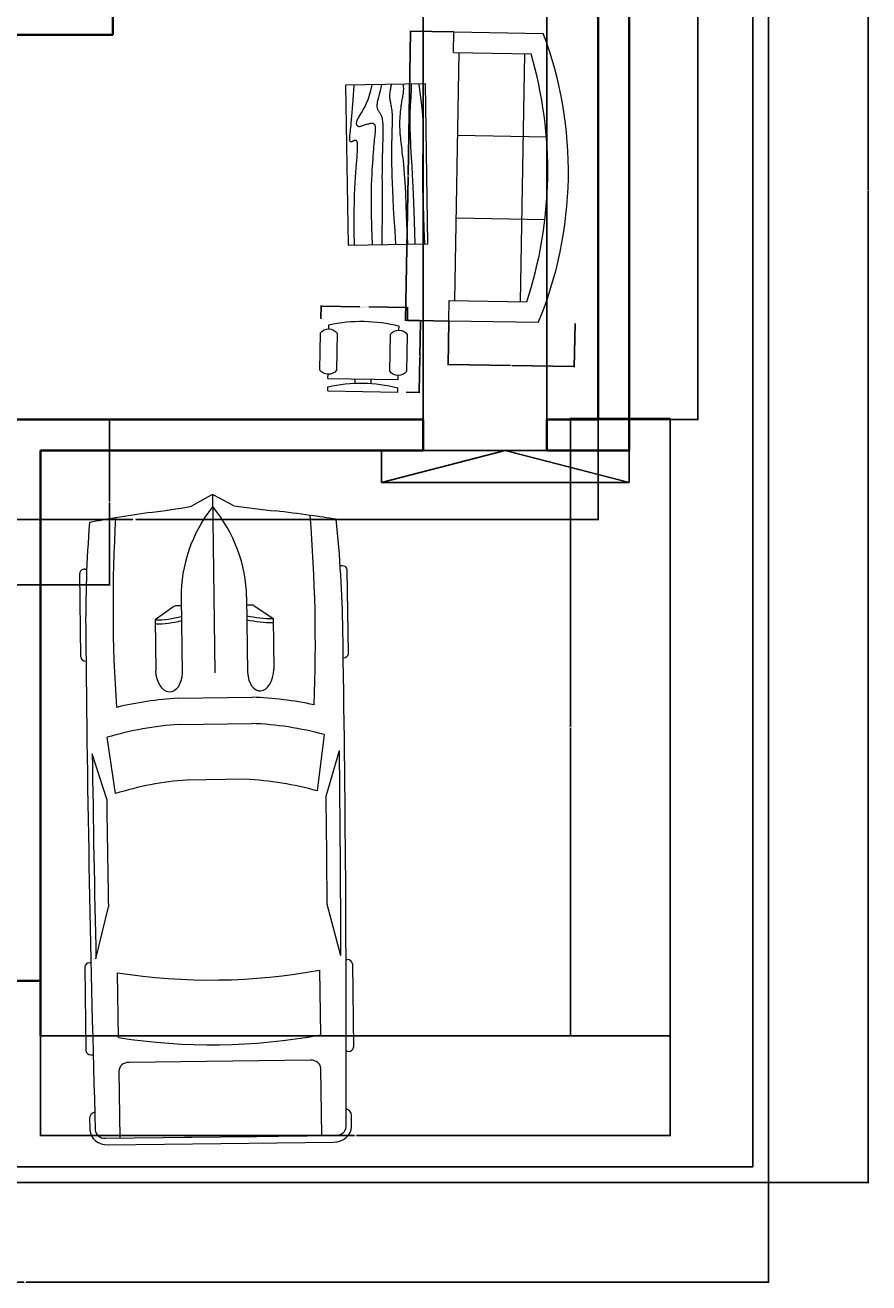
# Model space of a CAD drawing. Units: inches. Extents: x -1085 to 1941, y 1514 to 2348.
# Tile 3 of 9: x -613 to -367, y 1638 to 2003. Entities that reach past the tile are written whole.
import ezdxf

# ---------------------------------------------------------------- set-up
doc = ezdxf.new("R2010")
doc.units = ezdxf.units.IN
for name, color, linetype, lineweight in [('A-ANNO-DIMS', 2, 'Continuous', 18), ('A-FLOR-OTLN', 7, 'Continuous', 25), ('A-WALL', 7, 'Continuous', 35), ('C-PRKG-VEHS', 8, 'Continuous', 13), ('C-PROP', 8, 'Continuous', 25), ('FOUNITR-URE', 2, 'Continuous', 18)]:
    doc.layers.add(name, color=color, linetype=linetype, lineweight=lineweight)
doc.styles.get("Standard").update_dxf_attribs({"font": 'arial.ttf'})
doc.dimstyles.get("Standard").update_dxf_attribs({"dimtxt": 0.18, "dimasz": 0.18, "dimexe": 0.18, "dimexo": 0.0625, "dimgap": 0.09, "dimtad": 0, "dimtih": 1, "dimtoh": 1, "dimdec": 4, "dimzin": 0, "dimdsep": 46, "dimtxsty": 'Standard', "dimcen": 0.09, "dimadec": 0, "dimazin": 0, "dimtfac": 1, "dimtdec": 4, "dimtofl": 0, "dimtmove": 0, "dimatfit": 3, "dimfxl": 1, "dimtolj": 1, "dimtzin": 0, "dimarcsym": 0})

# ---------------------------------------------------------------- blocks, each defined once
blk = doc.blocks.new('Sofa - Roundback 7 ft.')
for p, q in [((-12.00002, -32.4421), (-12.00003, -6.5971)), ((11.99997, -32.4421), (11.99998, -6.5971)), ((-36.000027, -34), (-36.000027, -11.4696)), ((-35.999844, -13.3819), (35.9998, -13.3819)), ((35.99998, -34), (35.99998, -11.4696)), ((-36.000027, -32.4421), (35.99998, -32.4421))]:
    blk.add_line(p, q)
for points in [[(-36.000027, -34), (-42.000027, -34), (-42.000027, -8)], [(41.99998, -8), (41.99998, -34), (35.99998, -34)]]:
    blk.add_lwpolyline(points)
for centre, radius, start, end in [((0, -114.25), 114.25, 68.43141, 111.5686), ((-0.00001, -127.1968), 121.1968, 72.72033, 107.2797)]:
    blk.add_arc(centre, radius, start, end)
blk = doc.blocks.new('Chair - Desk')
for p, q in [((-8.5, 0), (-8.5, -1)), ((-8.5, 0), (8.5, 0)), ((8.5, 0), (8.5, -1)), ((-8.5, -3), (-8.5, -4)), ((-8.5, -3), (8.5, -3)), ((-2, -3), (-2, -1.9355)), ((2, -1.9576), (2, -3)), ((8.5, -3), (8.5, -4)), ((-10.5, -5), (-10.5, -14)), ((-6.5, -14), (-6.5, -5)), ((6.5, -5), (6.5, -14)), ((10.5, -14), (10.5, -5)), ((-8.5, -15), (-8.5, -16)), ((8.5, -15), (8.5, -16))]:
    blk.add_line(p, q)
for centre, radius, start, end in [((0, 34.625), 36.625, 256.5803, 283.4197), ((-8.5, -6.5), 2.5, 36.8699, 143.1301), ((8.5, -6.5), 2.5, 36.8699, 143.1301), ((-8.5, -12.5), 2.5, 216.8699, 323.1301), ((8.5, -12.5), 2.5, 216.8699, 323.1301), ((0, 19.625), 36.625, 256.5803, 283.4197)]:
    blk.add_arc(centre, radius, start, end)
blk = doc.blocks.new('*U28')
for p, q in [((536, 950.2), (536, 935.5)), ((1182.5, 987.8), (567.7, 987.8)), ((1214.1, 949.7), (1214.1, 950.2)), ((3440.5, 941.7), (3440.5, 950.2)), ((3472.1, 987.8), (4086.9, 987.8)), ((4118.5, 950.2), (4118.5, 934.1)), ((2234.8, 809.5), (1898.9, 912.4)), ((3411.6, 904.3), (3029.9, 807.2)), ((4736.4, -850.9), (4736.4, 850.9)), ((1778.8, 801), (2194.7, 745.5)), ((3515.9, 745.5), (3994.1, 745.5)), ((4736.4, 745.5), (4242, 745.5)), ((4785.3, -832.1), (4785.3, 832.1)), ((4178.7, 670.3), (4178.7, -670.3)), ((819.6, 295.3), (917.7, 436.1)), ((917.7, 436.1), (1293.8, 436.1)), ((815.9, 241.4), (815.9, 283.3)), ((756.2, 241.4), (1312.8, 241.4)), ((1496.5, -273.7), (1496.5, 273.7)), ((1690.4, -267.4), (1690.4, 267.4)), ((2101.5, 215.8), (2101.5, -215.8)), ((4736.4, -267.4), (4736.4, 267.4)), ((83, 155.7), (2.6, 10.3)), ((0, 0), (1312.8, 0)), ((2.6, -10.3), (83, -155.7)), ((756.2, -241.4), (1312.8, -241.4)), ((815.9, -241.4), (815.9, -283.3)), ((819.6, -295.3), (917.7, -436.1)), ((917.7, -436.1), (1293.8, -436.1)), ((2194.7, -745.5), (1778.8, -801)), ((2234.8, -809.5), (1898.9, -912.4)), ((3411.6, -904.3), (3029.9, -807.2)), ((3994.1, -745.5), (3515.9, -745.5)), ((4242, -745.5), (4736.4, -745.5)), ((536, -950.2), (536, -935.5)), ((1182.5, -987.8), (567.7, -987.8)), ((1214.1, -949.7), (1214.1, -950.2)), ((3440.5, -941.7), (3440.5, -950.2)), ((3472.1, -987.8), (4086.9, -987.8)), ((4118.5, -950.2), (4118.5, -934.1))]:
    blk.add_line(p, q)
for centre, major_axis, ratio, start_param, end_param in [((1046.3, -12467.9), (0, 13417.1), 0.842304, 0.00281, 0.075598), ((567.7, 950.2), (0, -37.6), 0.842304, 3.141593, 4.712389), ((1637.8, -268112.7), (0, 269062.9), 0.842304, -0.013397, 0.002797), ((1182.5, 950.2), (0, 37.6), 0.842304, -1.570796, 0), ((3472.1, 950.2), (0, -37.6), 0.842304, 3.141593, 4.712389), ((4086.9, 950.2), (0, 37.6), 0.842304, -1.570796, 0), ((4588, 910.3), (0, 56.4), 0.842304, -0.013017, 1.249894), ((1637.8, -268131.5), (0, 269121), 0.842304, -0.013397, -0.013017), ((4673.1, 832.1), (0, -133.3), 0.842304, 1.570796, 3.128196), ((6757.2, -699.1), (0, 7958), 0.842304, 1.367076, 1.39176), ((1637.8, -268112.7), (0, -269025.3), 0.842304, 3.133765, 3.140441), ((4673.1, 850.9), (0, -75.2), 0.842304, 1.570796, 3.128196), ((951.8, -15086.6), (0, -15832.5), 0.842304, 3.096046, 3.200911), ((3436.4, 136.8), (0, 2077), 0.842304, 1.245306, 1.50788), ((3799.7, 71.1), (0, -2021.3), 0.842304, 4.372215, 4.640744), ((2433, -93125.4), (0, -93935.2), 0.842304, 3.134049, 3.144098), ((433.9, 0), (0, 3734.3), 0.842304, 4.511394, 4.913384), ((912, 0), (0, 3734.3), 0.842304, 4.511394, 4.913384), ((4242, 670.3), (0, 75.2), 0.842304, 0, 1.570796), ((6583, -699.1), (0, -7754.7), 0.842304, 4.528606, 4.561838), ((3413.8, 136.8), (0, -2280.3), 0.842304, 4.449482, 4.652344), ((-5194.2, 1330.9), (0, -6374.4), 0.842304, 1.385369, 1.434372), ((331.1, 432), (0, 696.4), 0.842304, 4.435146, 4.718221), ((360.7, 432), (0, 696.4), 0.842304, 4.435146, 4.718221), ((1290.1, 338.8), (161, -9.1), 0.603834, -1.395552, 1.581315), ((831.8, 283.3), (0, 18.8), 0.842304, 0.879714, 1.570796), ((756.2, -1185.2), (0, 1426.7), 0.842304, 0, 0.590319), ((15.8, 0), (0, -18.8), 0.842304, 4.131459, 5.293319), ((756.2, 1185.2), (0, 1426.7), 0.842304, 2.551274, 3.141593), ((-5194.2, -1330.9), (0, 6374.4), 0.842304, -1.434372, -1.385369), ((331.1, -432), (0, -696.4), 0.842304, 1.564964, 1.848039), ((360.7, -432), (0, -696.4), 0.842304, 1.564964, 1.848039), ((3413.8, -136.8), (0, -2280.3), 0.842304, -1.510751, -1.307889), ((3436.4, -136.8), (0, -2077), 0.842304, -1.50788, -1.245306), ((3799.7, -71.1), (0, -2021.3), 0.842304, -1.499151, -1.230623), ((831.8, -283.3), (0, -18.8), 0.842304, 4.712389, 5.403472), ((6583, 699.1), (0, 7754.7), 0.842304, 1.721348, 1.754579), ((6757.2, 699.1), (0, 7958), 0.842304, 1.749832, 1.774517), ((951.8, 15086.6), (0, -15832.5), 0.842304, -0.059319, 0.045547), ((4242, -670.3), (0, -75.2), 0.842304, 4.712389, 6.283185), ((2433, 93125.4), (0, -93935.2), 0.842304, -0.002505, 0.007544), ((4673.1, -832.1), (0, -133.3), 0.842304, 0.013397, 1.570796), ((1046.3, 12467.9), (0, -13417.1), 0.842304, -0.075598, -0.00281), ((1637.8, 268112.7), (0, 269062.9), 0.842304, 3.138796, 3.15499), ((1637.8, 268112.7), (0, -269025.3), 0.842304, 0.001152, 0.007828), ((4673.1, -850.9), (0, 75.2), 0.842304, 3.15499, 4.712389), ((567.7, -950.2), (0, 37.6), 0.842304, 1.570796, 3.141593), ((1182.5, -950.2), (0, -37.6), 0.842304, 0, 1.570796), ((3472.1, -950.2), (0, -37.6), 0.842304, -1.570796, 0), ((4086.9, -950.2), (0, 37.6), 0.842304, 3.141593, 4.712389), ((4588, -910.3), (0, -56.4), 0.842304, -1.249894, 0.013017), ((1637.8, 268131.5), (0, 269121), 0.842304, 3.15461, 3.15499)]:
    blk.add_ellipse(centre, major_axis=major_axis, ratio=ratio, start_param=start_param, end_param=end_param)
at = {"extrusion": (0, 0, -1)}
blk.add_ellipse((1290.1, -338.8), major_axis=(161, 9.1), ratio=0.603834, start_param=-1.395552, end_param=1.581315, dxfattribs=at)
blk = doc.blocks.new('Table - Rectangular Woodgrain 60 x 30 in.')
for p, q in [((0, 0), (0, -30)), ((60, 0), (0, 0)), ((60, -30), (60, 0)), ((0, -30), (60, -30))]:
    blk.add_line(p, q)
for points in [[(0, -2.4), (4.8155, -2.418), (9.0302, -2.4688), (12.709, -2.5477), (15.9167, -2.65), (18.7181, -2.7711), (21.1781, -2.9063), (23.3616, -3.0508), (25.3333, -3.2), (27.1477, -3.3495), (28.8172, -3.4958), (30.3437, -3.636), (31.7291, -3.7667), (32.9756, -3.8849), (34.0849, -3.9875), (35.059, -4.0714), (35.9, -4.1334), (36.6114, -4.1711), (37.2041, -4.1854), (37.6906, -4.1779), (38.0833, -4.15), (38.3948, -4.1034), (38.6375, -4.0396), (38.8239, -3.9602), (38.9666, -3.8667), (39.0764, -3.7608), (39.1573, -3.6448), (39.2116, -3.521), (39.2416, -3.3917), (39.2498, -3.2593), (39.2385, -3.1261), (39.21, -2.9944), (39.1666, -2.8667), (39.111, -2.7447), (39.0468, -2.6281), (38.978, -2.5163), (38.9083, -2.4083), (38.8418, -2.3035), (38.7823, -2.201), (38.7337, -2.1001), (38.7, -2), (38.6844, -1.9003), (38.6875, -1.8021), (38.7094, -1.707), (38.75, -1.6167), (38.8094, -1.5326), (38.8875, -1.4563), (38.9844, -1.3893), (39.1, -1.3333), (39.2351, -1.2896), (39.3937, -1.2583), (39.5804, -1.2396), (39.8, -1.2333), (40.057, -1.2396), (40.3562, -1.2583), (40.7023, -1.2896), (41.1, -1.3333), (41.5547, -1.3895), (42.0755, -1.4573), (42.6721, -1.5361), (43.3542, -1.625), (44.1316, -1.7233), (45.014, -1.8302), (46.0114, -1.9449), (47.1333, -2.0667), (48.3862, -2.1947), (49.7625, -2.3281), (51.2513, -2.4663), (52.8416, -2.6083), (54.5226, -2.7535), (56.2833, -2.9011), (58.1127, -3.0501), (60, -3.2)], [(0, -9.2), (6.5759, -9.0858), (11.9385, -9.0365), (16.2527, -9.0418), (19.6833, -9.0917), (22.3952, -9.1759), (24.5531, -9.2844), (26.322, -9.4069), (27.8666, -9.5333), (29.3241, -9.6553), (30.7203, -9.7719), (32.0532, -9.8837), (33.3208, -9.9917), (34.5213, -10.0965), (35.6526, -10.199), (36.7128, -10.2999), (37.7, -10.4), (38.6129, -10.4996), (39.4531, -10.5969), (40.223, -10.6895), (40.925, -10.775), (41.5613, -10.8512), (42.1344, -10.9156), (42.6465, -10.966), (43.1, -11), (43.4976, -11.0158), (43.8437, -11.0136), (44.143, -10.9942), (44.4, -10.9583), (44.6195, -10.9069), (44.8062, -10.8406), (44.9648, -10.7603), (45.1, -10.6667), (45.2155, -10.5598), (45.3114, -10.4365), (45.3871, -10.2929), (45.4416, -10.125), (45.4743, -9.929), (45.4844, -9.7011), (45.4709, -9.4371), (45.4333, -9.1333), (45.3716, -8.7883), (45.2896, -8.4104), (45.1919, -8.0107), (45.0833, -7.6), (44.9685, -7.1893), (44.8521, -6.7896), (44.7388, -6.4117), (44.6333, -6.0667), (44.54, -5.7628), (44.4614, -5.4979), (44.4001, -5.2675), (44.3583, -5.0667), (44.3384, -4.8909), (44.3427, -4.7354), (44.3736, -4.5956), (44.4333, -4.4667), (44.5236, -4.3453), (44.6427, -4.2333), (44.7884, -4.1339), (44.9583, -4.05), (45.1501, -3.9849), (45.3614, -3.9417), (45.59, -3.9234), (45.8333, -3.9333), (46.0915, -3.9749), (46.3734, -4.0531), (46.6906, -4.1736), (47.0542, -4.3417), (47.4756, -4.5629), (47.9661, -4.8427), (48.5372, -5.1866), (49.2, -5.6), (49.9676, -6.0844), (50.8594, -6.625), (51.8965, -7.2031), (53.1, -7.8), (54.491, -8.3969), (56.0906, -8.975), (57.9199, -9.5156), (60, -10)], [(0, -12.8), (5.1847, -12.9322), (9.6213, -13.0323), (13.3963, -13.1059), (16.5958, -13.1583), (19.3063, -13.1952), (21.614, -13.2219), (23.6054, -13.2439), (25.3666, -13.2667), (26.9728, -13.2947), (28.4531, -13.3281), (29.8256, -13.3663), (31.1083, -13.4083), (32.3191, -13.4535), (33.476, -13.501), (34.597, -13.5501), (35.7, -13.6), (36.7984, -13.6497), (37.8875, -13.6979), (38.9578, -13.743), (40, -13.7833), (41.0047, -13.8174), (41.9625, -13.8438), (42.864, -13.8607), (43.7, -13.8667), (44.4631, -13.8604), (45.1552, -13.8417), (45.7801, -13.8104), (46.3416, -13.7667), (46.8439, -13.7104), (47.2906, -13.6417), (47.6858, -13.5604), (48.0333, -13.4667), (48.3375, -13.3608), (48.6042, -13.2448), (48.8396, -13.121), (49.05, -12.9917), (49.2417, -12.8593), (49.4208, -12.7261), (49.5937, -12.5944), (49.7667, -12.4667), (49.9452, -12.3451), (50.1323, -12.2313), (50.3303, -12.1268), (50.5416, -12.0333), (50.7686, -11.9524), (51.0135, -11.8854), (51.2788, -11.8341), (51.5666, -11.8), (51.8785, -11.7843), (52.2116, -11.7865), (52.562, -11.8059), (52.926, -11.8417), (53.2998, -11.8931), (53.6795, -11.9594), (54.0614, -12.0397), (54.4416, -12.1333), (54.8223, -12.2401), (55.2293, -12.3625), (55.6942, -12.5037), (56.2489, -12.6667), (56.9251, -12.8547), (57.7545, -13.0708), (58.7689, -13.3182), (60, -13.6)], [(0, -18), (5.124, -17.7273), (9.6609, -17.5057), (13.6705, -17.3303), (17.2125, -17.1958), (20.3467, -17.0973), (23.1328, -17.0297), (25.6307, -16.9878), (27.9, -16.9667), (29.9928, -16.9617), (31.9302, -16.9703), (33.7254, -16.9907), (35.3917, -17.0208), (36.9423, -17.0588), (38.3906, -17.1026), (39.7499, -17.1503), (41.0333, -17.2), (42.2519, -17.2496), (43.4073, -17.2969), (44.4986, -17.3395), (45.525, -17.375), (46.4858, -17.4012), (47.3802, -17.4156), (48.2074, -17.416), (48.9667, -17.4), (49.6583, -17.3662), (50.2872, -17.3167), (50.8595, -17.2547), (51.3812, -17.1833), (51.8584, -17.1057), (52.2971, -17.025), (52.7034, -16.9443), (53.0833, -16.8667), (53.443, -16.7951), (53.789, -16.7313), (54.128, -16.6768), (54.4666, -16.6334), (54.8115, -16.6024), (55.1693, -16.5854), (55.5465, -16.5841), (55.95, -16.6), (56.3828, -16.6337), (56.8346, -16.6823), (57.2915, -16.7418), (57.7396, -16.8084), (58.165, -16.878), (58.5539, -16.9469), (58.8924, -17.0111), (59.1666, -17.0667), (59.3679, -17.1107), (59.5078, -17.1438), (59.6032, -17.1675), (59.6708, -17.1833), (59.7275, -17.193), (59.7901, -17.1979), (59.8753, -17.1998), (60, -17.2)], [(0, -22.4), (8.0098, -22.2501), (14.4094, -22.1011), (19.4168, -21.9535), (23.25, -21.8083), (26.1269, -21.6663), (28.2656, -21.5281), (29.884, -21.3947), (31.2, -21.2667), (32.3967, -21.1448), (33.5172, -21.0292), (34.5697, -20.9198), (35.5625, -20.8167), (36.5037, -20.7198), (37.4015, -20.6292), (38.2642, -20.5448), (39.1, -20.4667), (39.9164, -20.3951), (40.7187, -20.3313), (41.5117, -20.2768), (42.3, -20.2333), (43.0883, -20.2024), (43.8812, -20.1854), (44.6836, -20.1841), (45.5, -20.2), (46.3328, -20.234), (47.1747, -20.2844), (48.0163, -20.3488), (48.8479, -20.425), (49.66, -20.5106), (50.4429, -20.6031), (51.1872, -20.7004), (51.8833, -20.8), (52.5246, -20.8999), (53.1166, -20.9995), (53.6681, -21.0983), (54.1875, -21.1958), (54.6834, -21.2919), (55.1646, -21.3859), (55.6394, -21.4777), (56.1167, -21.5667), (56.6028, -21.6515), (57.0961, -21.7266), (57.5929, -21.7852), (58.0896, -21.8208), (58.5823, -21.8268), (59.0674, -21.7964), (59.5412, -21.723), (60, -21.6)], [(0, -25.2), (8.6355, -25.0504), (15.7026, -24.9031), (21.4049, -24.7606), (25.9458, -24.625), (29.529, -24.4988), (32.3578, -24.3844), (34.6359, -24.284), (36.5667, -24.2), (38.3213, -24.1341), (39.9417, -24.0854), (41.437, -24.0523), (42.8167, -24.0333), (44.0901, -24.0268), (45.2667, -24.0313), (46.3557, -24.0451), (47.3667, -24.0667), (48.309, -24.0947), (49.1928, -24.1287), (50.0284, -24.168), (50.826, -24.2125), (51.5959, -24.2617), (52.3483, -24.3151), (53.0935, -24.3725), (53.8417, -24.4334), (54.6009, -24.497), (55.3699, -24.561), (56.1454, -24.6226), (56.9239, -24.6792), (57.7021, -24.7279), (58.4764, -24.7662), (59.2435, -24.7911), (60, -24.8)], [(0, -28.8), (5.6867, -28.6681), (10.45, -28.5698), (14.407, -28.5012), (17.675, -28.4584), (20.3711, -28.4374), (22.6125, -28.4344), (24.5164, -28.4455), (26.2, -28.4667), (27.762, -28.4947), (29.2276, -28.5281), (30.6033, -28.5663), (31.8958, -28.6084), (33.1118, -28.6535), (34.2578, -28.7011), (35.3405, -28.7501), (36.3666, -28.8), (37.3443, -28.8497), (38.288, -28.8974), (39.2137, -28.9412), (40.1375, -28.9792), (41.0753, -29.0093), (42.0432, -29.0297), (43.0572, -29.0384), (44.1333, -29.0333), (45.2936, -29.0114), (46.5843, -28.9641), (48.0579, -28.8816), (49.7666, -28.7542), (51.7629, -28.5721), (54.0989, -28.3255), (56.8272, -28.0048), (60, -27.6)]]:
    blk.add_lwpolyline(points)
blk = doc.blocks.new('*D42')
at = {"layer": 'A-ANNO-DIMS', "color": 0, "lineweight": -2, "transparency": 16777216}
for p, q in [((-500.6, 2001.04), (-501.33, 1959.41)), ((-488.06, 2001), (-500.78, 2001.22)), ((-502.05, 1917.41), (-501.33, 1959.04)), ((-489.52, 1917.01), (-502.24, 1917.23))]:
    blk.add_line(p, q, dxfattribs=at)
at = {"layer": 'A-ANNO-DIMS', "color": 0, "transparency": 16777216}
for points in [[(-500.63, 2001.04), (-500.57, 2001.04), (-500.6, 2001.22)], [(-502.08, 1917.41), (-502.02, 1917.41), (-502.06, 1917.23)]]:
    blk.add_solid(points, dxfattribs=at)
at = {"layer": 'Defpoints', "color": 0, "transparency": 16777216}
for p in [(-488, 2001), (-502.06, 1917.23), (-489.46, 1917.01)]:
    blk.add_point(p, dxfattribs=at)
at = {"layer": 'A-ANNO-DIMS', "color": 0, "transparency": 16777216, "insert": (-501.33, 1959.22), "char_height": 0.18, "attachment_point": 5}
blk.add_mtext('\\A1;SOFA 84', dxfattribs=at)
blk = doc.blocks.new('*D43')
at = {"layer": 'A-ANNO-DIMS', "color": 0, "lineweight": -2, "transparency": 16777216}
for p, q in [((-489.46, 1916.95), (-489.68, 1904.23)), ((-452.8, 1916.31), (-453.02, 1903.6)), ((-489.5, 1904.41), (-471.57, 1904.1)), ((-453.2, 1903.78), (-471.13, 1904.09))]:
    blk.add_line(p, q, dxfattribs=at)
at = {"layer": 'A-ANNO-DIMS', "color": 0, "transparency": 16777216}
for points in [[(-489.5, 1904.44), (-489.5, 1904.38), (-489.68, 1904.41)], [(-453.2, 1903.81), (-453.2, 1903.75), (-453.02, 1903.78)]]:
    blk.add_solid(points, dxfattribs=at)
at = {"layer": 'Defpoints', "color": 0, "transparency": 16777216}
for p in [(-489.46, 1917.01), (-452.8, 1916.37), (-453.02, 1903.78)]:
    blk.add_point(p, dxfattribs=at)
at = {"layer": 'A-ANNO-DIMS', "color": 0, "transparency": 16777216, "insert": (-471.35, 1904.09), "char_height": 0.18, "attachment_point": 5}
blk.add_mtext('\\A1;37', dxfattribs=at)
blk = doc.blocks.new('*D56')
at = {"layer": 'A-ANNO-DIMS', "color": 0, "lineweight": -2, "transparency": 16777216}
for p, q in [((-526.68, 1917.64), (-526.61, 1921.53)), ((-526.43, 1921.35), (-515.36, 1921.15)), ((-501.63, 1920.91), (-512.7, 1921.1)), ((-501.51, 1917.19), (-501.45, 1921.08))]:
    blk.add_line(p, q, dxfattribs=at)
at = {"layer": 'A-ANNO-DIMS', "color": 0, "transparency": 16777216}
for points in [[(-526.43, 1921.38), (-526.43, 1921.32), (-526.61, 1921.35)], [(-501.63, 1920.94), (-501.63, 1920.88), (-501.45, 1920.9)]]:
    blk.add_solid(points, dxfattribs=at)
at = {"layer": 'Defpoints', "color": 0, "transparency": 16777216}
for p in [(-526.68, 1917.58), (-501.45, 1920.9), (-501.52, 1917.13)]:
    blk.add_point(p, dxfattribs=at)
at = {"layer": 'A-ANNO-DIMS', "color": 0, "transparency": 16777216, "insert": (-514.03, 1921.13), "char_height": 0.18, "attachment_point": 5}
blk.add_mtext('\\A1;DESK CHAIR 25 TYP.', dxfattribs=at)
blk = doc.blocks.new('*D57')
at = {"layer": 'A-ANNO-DIMS', "color": 0, "lineweight": -2, "transparency": 16777216}
for p, q in [((-501.45, 1917.13), (-497.56, 1917.06)), ((-497.74, 1916.88), (-497.92, 1906.86)), ((-498.11, 1896.47), (-497.93, 1906.5)), ((-501.82, 1896.36), (-497.93, 1896.29))]:
    blk.add_line(p, q, dxfattribs=at)
at = {"layer": 'A-ANNO-DIMS', "color": 0, "transparency": 16777216}
for points in [[(-497.77, 1916.88), (-497.71, 1916.88), (-497.74, 1917.06)], [(-498.14, 1896.47), (-498.08, 1896.47), (-498.11, 1896.29)]]:
    blk.add_solid(points, dxfattribs=at)
at = {"layer": 'Defpoints', "color": 0, "transparency": 16777216}
for p in [(-501.52, 1917.13), (-501.88, 1896.36), (-498.11, 1896.29)]:
    blk.add_point(p, dxfattribs=at)
at = {"layer": 'A-ANNO-DIMS', "color": 0, "transparency": 16777216, "insert": (-497.93, 1906.68), "char_height": 0.18, "attachment_point": 5}
blk.add_mtext('\\A1;21 TYP.', dxfattribs=at)
blk = doc.blocks.new('*D94')
at = {"layer": 'A-ANNO-DIMS', "color": 0, "lineweight": -2, "transparency": 16777216}
for p, q in [((-828.6, 1666.82), (-828.6, 1637.7)), ((-396.6, 1666.82), (-396.6, 1637.7)), ((-828.42, 1637.88), (-612.89, 1637.88)), ((-396.78, 1637.88), (-612.31, 1637.88))]:
    blk.add_line(p, q, dxfattribs=at)
at = {"layer": 'A-ANNO-DIMS', "color": 0, "transparency": 16777216}
for points in [[(-828.42, 1637.91), (-828.42, 1637.85), (-828.6, 1637.88)], [(-396.78, 1637.91), (-396.78, 1637.85), (-396.6, 1637.88)]]:
    blk.add_solid(points, dxfattribs=at)
at = {"layer": 'Defpoints', "color": 0, "transparency": 16777216}
for p in [(-828.6, 1666.88), (-396.6, 1666.88), (-396.6, 1637.88)]:
    blk.add_point(p, dxfattribs=at)
at = {"layer": 'A-ANNO-DIMS', "color": 0, "transparency": 16777216, "insert": (-612.6, 1637.88), "char_height": 0.18, "attachment_point": 5}
blk.add_mtext('\\A1;432', dxfattribs=at)
blk = doc.blocks.new('*D95')
at = {"layer": 'A-ANNO-DIMS', "color": 0, "lineweight": -2, "transparency": 16777216}
for p, q in [((-396.54, 2242.88), (-367.42, 2242.88)), ((-367.6, 2242.7), (-367.6, 1955.07)), ((-367.6, 1667.06), (-367.6, 1954.7)), ((-396.54, 1666.88), (-367.42, 1666.88))]:
    blk.add_line(p, q, dxfattribs=at)
at = {"layer": 'A-ANNO-DIMS', "color": 0, "transparency": 16777216}
for points in [[(-367.63, 2242.7), (-367.57, 2242.7), (-367.6, 2242.88)], [(-367.63, 1667.06), (-367.57, 1667.06), (-367.6, 1666.88)]]:
    blk.add_solid(points, dxfattribs=at)
at = {"layer": 'Defpoints', "color": 0, "transparency": 16777216}
for p in [(-396.6, 2242.88), (-367.6, 2242.88), (-396.6, 1666.88)]:
    blk.add_point(p, dxfattribs=at)
at = {"layer": 'A-ANNO-DIMS', "color": 0, "transparency": 16777216, "insert": (-367.6, 1954.88), "char_height": 0.18, "attachment_point": 5}
blk.add_mtext('\\A1;576', dxfattribs=at)
blk = doc.blocks.new('*D108')
at = {"layer": 'A-ANNO-DIMS', "color": 0, "lineweight": -2, "transparency": 16777216}
for p, q in [((-496.94, 1888.45), (-496.94, 2272.06)), ((-496.76, 2271.88), (-479.16, 2271.88)), ((-461.12, 2271.88), (-478.72, 2271.88)), ((-460.94, 1888.45), (-460.94, 2272.06))]:
    blk.add_line(p, q, dxfattribs=at)
at = {"layer": 'A-ANNO-DIMS', "color": 0, "transparency": 16777216}
for points in [[(-496.76, 2271.91), (-496.76, 2271.85), (-496.94, 2271.88)], [(-461.12, 2271.91), (-461.12, 2271.85), (-460.94, 2271.88)]]:
    blk.add_solid(points, dxfattribs=at)
at = {"layer": 'Defpoints', "color": 0, "transparency": 16777216}
for p in [(-460.94, 2271.88), (-496.94, 1888.38), (-460.94, 1888.38)]:
    blk.add_point(p, dxfattribs=at)
at = {"layer": 'A-ANNO-DIMS', "color": 0, "transparency": 16777216, "insert": (-478.94, 2271.88), "char_height": 0.18, "attachment_point": 5}
blk.add_mtext('\\A1;36', dxfattribs=at)
blk = doc.blocks.new('*D110')
at = {"layer": 'A-ANNO-DIMS', "color": 0, "lineweight": -2, "transparency": 16777216}
for p, q in [((-446.04, 2196.38), (-416.92, 2196.38)), ((-417.1, 2196.2), (-417.1, 2042.57)), ((-417.1, 1888.56), (-417.1, 2042.2)), ((-446.04, 1888.38), (-416.92, 1888.38))]:
    blk.add_line(p, q, dxfattribs=at)
at = {"layer": 'A-ANNO-DIMS', "color": 0, "transparency": 16777216}
for points in [[(-417.13, 2196.2), (-417.07, 2196.2), (-417.1, 2196.38)], [(-417.13, 1888.56), (-417.07, 1888.56), (-417.1, 1888.38)]]:
    blk.add_solid(points, dxfattribs=at)
at = {"layer": 'Defpoints', "color": 0, "transparency": 16777216}
for p in [(-446.1, 2196.38), (-446.1, 1888.38), (-417.1, 1888.38)]:
    blk.add_point(p, dxfattribs=at)
at = {"layer": 'A-ANNO-DIMS', "color": 0, "transparency": 16777216, "insert": (-417.1, 2042.38), "char_height": 0.18, "attachment_point": 5}
blk.add_mtext('\\A1;308', dxfattribs=at)
blk = doc.blocks.new('*D112')
at = {"layer": 'A-ANNO-DIMS', "color": 0, "lineweight": -2, "transparency": 16777216}
for p, q in [((-715.62, 1888.32), (-715.62, 1859.2)), ((-446.1, 1888.32), (-446.1, 1859.2)), ((-715.44, 1859.38), (-581.26, 1859.38)), ((-446.28, 1859.38), (-580.47, 1859.38))]:
    blk.add_line(p, q, dxfattribs=at)
at = {"layer": 'A-ANNO-DIMS', "color": 0, "transparency": 16777216}
for points in [[(-715.44, 1859.41), (-715.44, 1859.35), (-715.62, 1859.38)], [(-446.28, 1859.41), (-446.28, 1859.35), (-446.1, 1859.38)]]:
    blk.add_solid(points, dxfattribs=at)
at = {"layer": 'Defpoints', "color": 0, "transparency": 16777216}
for p in [(-715.62, 1888.38), (-446.1, 1888.38), (-715.62, 1859.38)]:
    blk.add_point(p, dxfattribs=at)
at = {"layer": 'A-ANNO-DIMS', "color": 0, "transparency": 16777216, "insert": (-580.86, 1859.38), "char_height": 0.18, "attachment_point": 5}
blk.add_mtext('\\A1;269.5', dxfattribs=at)
blk = doc.blocks.new('*D113')
at = {"layer": 'A-ANNO-DIMS', "color": 0, "lineweight": -2, "transparency": 16777216}
for p, q in [((-608.1, 1709.42), (-608.1, 1680.3)), ((-425.1, 1709.42), (-425.1, 1680.3)), ((-607.92, 1680.48), (-516.88, 1680.48)), ((-425.28, 1680.48), (-516.32, 1680.48))]:
    blk.add_line(p, q, dxfattribs=at)
at = {"layer": 'A-ANNO-DIMS', "color": 0, "transparency": 16777216}
for points in [[(-607.92, 1680.51), (-607.92, 1680.45), (-608.1, 1680.48)], [(-425.28, 1680.51), (-425.28, 1680.45), (-425.1, 1680.48)]]:
    blk.add_solid(points, dxfattribs=at)
at = {"layer": 'Defpoints', "color": 0, "transparency": 16777216}
for p in [(-608.1, 1709.48), (-425.1, 1709.48), (-608.1, 1680.48)]:
    blk.add_point(p, dxfattribs=at)
at = {"layer": 'A-ANNO-DIMS', "color": 0, "transparency": 16777216, "insert": (-516.6, 1680.48), "char_height": 0.18, "attachment_point": 5}
blk.add_mtext('\\A1;183', dxfattribs=at)
blk = doc.blocks.new('*D114')
at = {"layer": 'A-ANNO-DIMS', "color": 0, "lineweight": -2, "transparency": 16777216}
for p, q in [((-425.17, 1888.71), (-454.28, 1888.71)), ((-454.1, 1888.53), (-454.1, 1799.28)), ((-454.1, 1709.66), (-454.1, 1798.91)), ((-425.17, 1709.48), (-454.28, 1709.48))]:
    blk.add_line(p, q, dxfattribs=at)
at = {"layer": 'A-ANNO-DIMS', "color": 0, "transparency": 16777216}
for points in [[(-454.13, 1888.53), (-454.07, 1888.53), (-454.1, 1888.71)], [(-454.13, 1709.66), (-454.07, 1709.66), (-454.1, 1709.48)]]:
    blk.add_solid(points, dxfattribs=at)
at = {"layer": 'Defpoints', "color": 0, "transparency": 16777216}
for p in [(-454.1, 1888.71), (-425.1, 1888.71), (-425.1, 1709.48)]:
    blk.add_point(p, dxfattribs=at)
at = {"layer": 'A-ANNO-DIMS', "color": 0, "transparency": 16777216, "insert": (-454.1, 1799.09), "char_height": 0.18, "attachment_point": 5}
blk.add_mtext('\\A1;179.23', dxfattribs=at)
blk = doc.blocks.new('*D118')
at = {"layer": 'A-ANNO-DIMS', "color": 0, "lineweight": -2, "transparency": 16777216}
for p, q in [((-617.04, 1888.38), (-587.92, 1888.38)), ((-588.1, 1888.2), (-588.1, 1864.57)), ((-588.1, 1840.56), (-588.1, 1864.2)), ((-617.04, 1840.38), (-587.92, 1840.38))]:
    blk.add_line(p, q, dxfattribs=at)
at = {"layer": 'A-ANNO-DIMS', "color": 0, "transparency": 16777216}
for points in [[(-588.13, 1888.2), (-588.07, 1888.2), (-588.1, 1888.38)], [(-588.13, 1840.56), (-588.07, 1840.56), (-588.1, 1840.38)]]:
    blk.add_solid(points, dxfattribs=at)
at = {"layer": 'Defpoints', "color": 0, "transparency": 16777216}
for p in [(-617.1, 1888.38), (-617.1, 1840.38), (-588.1, 1840.38)]:
    blk.add_point(p, dxfattribs=at)
at = {"layer": 'A-ANNO-DIMS', "color": 0, "transparency": 16777216, "insert": (-588.1, 1864.38), "char_height": 0.18, "attachment_point": 5}
blk.add_mtext('\\A1;48', dxfattribs=at)

msp = doc.modelspace()

# ---------------------------------------------------------------- linework, layer by layer
at = {"layer": 'A-FLOR-OTLN'}
for p, q in [((-425.1032, 1888.7098), (-437.1032, 1888.7098)), ((-425.1032, 1879.3835), (-425.1032, 1888.7098)), ((-437.1032, 1879.3835), (-509.0632, 1879.3835)), ((-509.0632, 1879.3835), (-509.0632, 1870.0845)), ((-473.0832, 1879.3835), (-509.0632, 1870.0845)), ((-509.0632, 1870.0845), (-473.0832, 1879.3835)), ((-473.0832, 1879.3835), (-437.1032, 1870.0845)), ((-437.1032, 1879.3835), (-437.1032, 1870.0845)), ((-425.1032, 1709.4784), (-425.1032, 1879.3835)), ((-509.0632, 1870.0845), (-437.4691, 1870.0845)), ((-437.4691, 1870.0845), (-437.1032, 1870.0845)), ((-437.1032, 1709.4784), (-608.1032, 1709.4784)), ((-437.1032, 1709.4784), (-425.1032, 1709.4784)), ((-608.1032, 1671.3835), (-608.1032, 1671.3835))]:
    msp.add_line(p, q, dxfattribs=at)
at = {"layer": 'A-WALL'}
for p, q in [((-437.1032, 2205.3835), (-437.1032, 1888.7098)), ((-446.1032, 2196.3835), (-446.1032, 1888.3835)), ((-587.1032, 2000.1777), (-587.1032, 2129.054)), ((-645.6032, 2000.1777), (-591.6032, 2000.1777)), ((-591.6032, 2000.1777), (-587.1032, 2000.1777)), ((-617.1032, 1888.3835), (-496.941, 1888.3835)), ((-496.941, 1879.3835), (-496.941, 1888.3835)), ((-460.941, 1888.3835), (-460.941, 1879.3835)), ((-460.941, 1888.3835), (-446.1032, 1888.3835)), ((-437.1032, 1888.7098), (-437.1032, 1879.3835)), ((-608.1032, 1709.4784), (-608.1032, 1879.3835)), ((-608.1032, 1879.3835), (-496.941, 1879.3835)), ((-460.941, 1879.3835), (-446.1032, 1879.3835)), ((-446.1032, 1879.3835), (-437.1032, 1879.3835)), ((-608.1032, 1734.3835), (-608.1032, 1709.4784)), ((-608.1032, 1725.3835), (-791.1032, 1725.3835)), ((-608.1032, 1725.3835), (-608.1032, 1709.4784))]:
    msp.add_line(p, q, dxfattribs=at)
at = {"layer": 'C-PROP'}
for p, q in [((-396.6032, 2242.8835), (-396.6032, 1666.8835)), ((-401.1032, 2238.3835), (-401.1032, 1671.3835)), ((-401.1032, 1671.3835), (-824.1032, 1671.3835)), ((-396.6032, 1666.8835), (-828.6032, 1666.8835))]:
    msp.add_line(p, q, dxfattribs=at)

# ---------------------------------------------------------------- block references
at = {"layer": 'C-PRKG-VEHS', "xscale": 0.0393700787401575, "yscale": 0.0393700787401575, "zscale": 0.0393700787401575, "rotation": 270.7362034403327}
msp.add_blockref('*U28', (-558.1441, 1866.5654), dxfattribs=at)
at = {"layer": 'FOUNITR-URE', "rotation": 269.0061411650281}
msp.add_blockref('Sofa - Roundback 7 ft.', (-454.7353, 1958.414), dxfattribs=at)
at = {"layer": 'FOUNITR-URE'}
for name, p, xscale, yscale, zscale, rotation in [('Table - Rectangular Woodgrain 60 x 30 in.', (-518.7526, 1939.0819), 0.7739415990810241, 0.7739415990810241, 0.7739415990810241, 90.90402502805208), ('Chair - Desk', (-514.4677, 1896.5807), -1.198560681527003, 1.198560681527003, 1.198560681527003, 178.9819179435781)]:
    msp.add_blockref(name, p, dxfattribs=dict(at, xscale=xscale, yscale=yscale, zscale=zscale, rotation=rotation))

# ---------------------------------------------------------------- dimensions: what is measured, and where the dimension line sits
at = {"layer": 'A-ANNO-DIMS'}
for base, p1, p2, picture, middle in [((-460.941, 2271.8835), (-496.941, 1888.3835), (-460.941, 1888.3835), '*D108', (-478.941, 2271.8835)), ((-396.6032, 1637.8835), (-828.6032, 1666.8835), (-396.6032, 1666.8835), '*D94', (-612.6032, 1637.8835))]:
    dim = msp.add_linear_dim(base=base, p1=p1, p2=p2, dimstyle='Standard', override={"dimdec": 0, "dimlfac": 1, "dimrnd": 0, "dimzin": 0, "dimdsep": 46, "dimlunit": 2}, dxfattribs=at)
    dim.commit()
    dim.dimension.update_dxf_attribs({"geometry": picture, "text_midpoint": middle})
for base, p1, p2, angle, override, picture, middle in [((-367.6032, 2242.8835), (-396.6032, 1666.8835), (-396.6032, 2242.8835), 90, {"dimdec": 0, "dimlfac": 1, "dimrnd": 0, "dimzin": 0, "dimdsep": 46, "dimlunit": 2}, '*D95', (-367.6032, 1954.8835)), ((-417.1032, 1888.3835), (-446.1032, 2196.3835), (-446.1032, 1888.3835), 270, {"dimdec": 0, "dimlfac": 1, "dimrnd": 0, "dimzin": 0, "dimdsep": 46, "dimlunit": 2}, '*D110', (-417.1032, 2042.3835)), ((-453.0161, 1903.7759), (-489.4587, 1917.01), (-452.7975, 1916.374), 359.006141, {"dimdec": 0, "dimlfac": 1, "dimrnd": 0, "dimzin": 0, "dimdsep": 46, "dimlunit": 2}, '*D43', (-471.3467, 1904.0939)), ((-715.6221, 1859.3835), (-446.1032, 1888.3835), (-715.6221, 1888.3835), 180, {"dimdec": 1, "dimlfac": 1, "dimrnd": 0, "dimzin": 0, "dimdsep": 46, "dimlunit": 2}, '*D112', (-580.8627, 1859.3835)), ((-588.1032, 1840.3835), (-617.1032, 1888.3835), (-617.1032, 1840.3835), 270, {"dimdec": 0, "dimlfac": 1, "dimrnd": 0, "dimzin": 0, "dimdsep": 46, "dimlunit": 2}, '*D118', (-588.1032, 1864.3835)), ((-454.1032, 1888.7098), (-425.1032, 1709.4784), (-425.1032, 1888.7098), 90, {"dimdec": 2, "dimlfac": 1, "dimrnd": 0, "dimzin": 0, "dimdsep": 46, "dimlunit": 2}, '*D114', (-454.1032, 1799.0941)), ((-608.1032, 1680.4784), (-425.1032, 1709.4784), (-608.1032, 1709.4784), 180, {"dimdec": 0, "dimlfac": 1, "dimrnd": 0, "dimzin": 0, "dimdsep": 46, "dimlunit": 2}, '*D113', (-516.6032, 1680.4784))]:
    dim = msp.add_linear_dim(base=base, p1=p1, p2=p2, angle=angle, dimstyle='Standard', override=override, dxfattribs=at)
    dim.commit()
    dim.dimension.update_dxf_attribs({"geometry": picture, "text_midpoint": middle})
for base, p1, p2, angle, text, picture, middle in [((-502.0568, 1917.2286), (-488.0017, 2000.9974), (-489.4587, 1917.01), 269.006141, 'SOFA <>', '*D42', (-501.3283, 1959.2223)), ((-501.4486, 1920.9037), (-526.6815, 1917.5761), (-501.5157, 1917.1289), 358.981918, 'DESK CHAIR <> TYP.', '*D56', (-514.0315, 1921.1273)), ((-498.11, 1896.29), (-501.5157, 1917.1289), (-501.8848, 1896.3571), 268.981918, '<> TYP.', '*D57', (-497.9254, 1906.6759))]:
    dim = msp.add_linear_dim(base=base, p1=p1, p2=p2, angle=angle, text=text, dimstyle='Standard', override={"dimdec": 0, "dimlfac": 1, "dimrnd": 0, "dimzin": 0, "dimdsep": 46, "dimlunit": 2}, dxfattribs=at)
    dim.commit()
    dim.dimension.update_dxf_attribs({"geometry": picture, "text_midpoint": middle})

doc.saveas('drawing.dxf')
